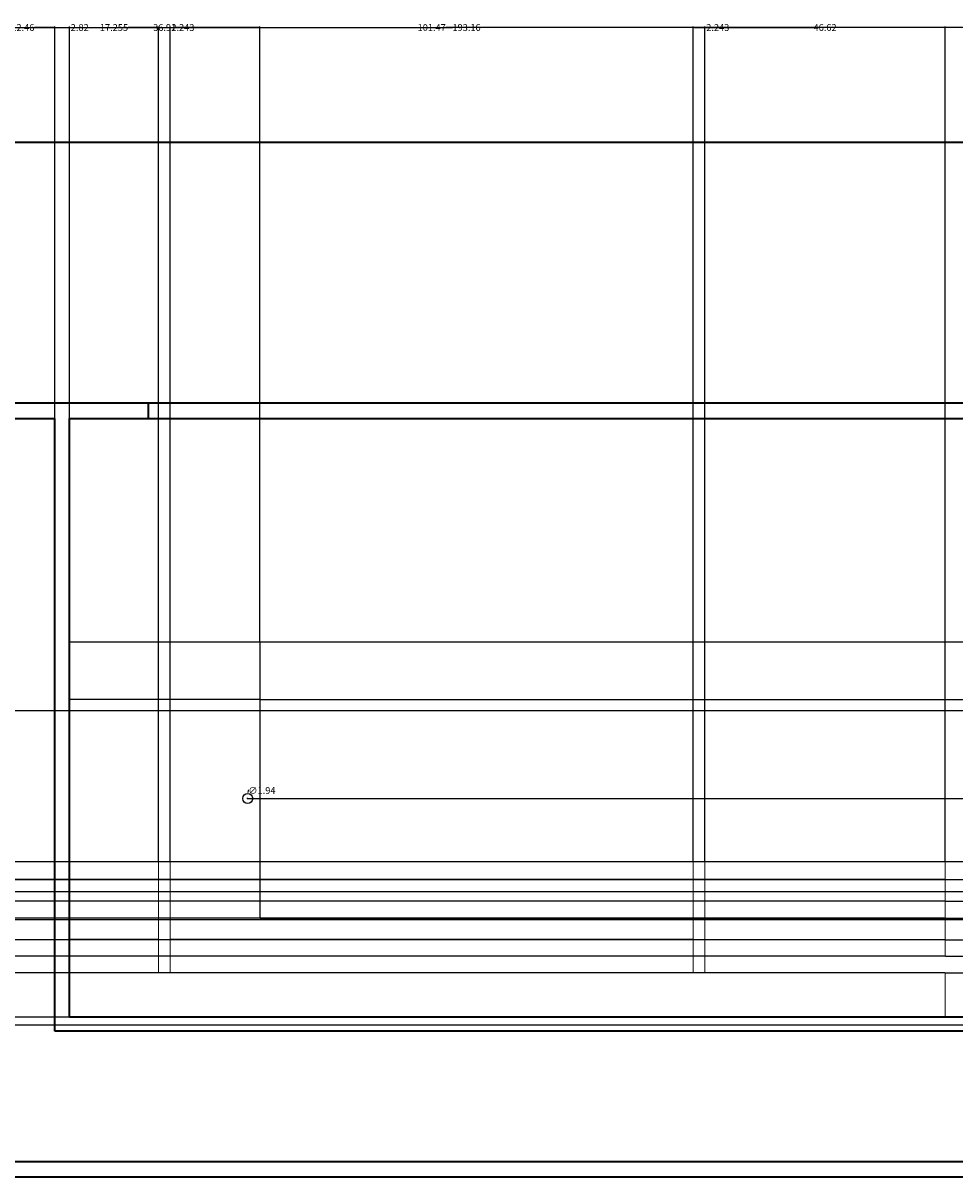
# Model space of a CAD drawing. Units: inches. Extents: x 30 to 515, y 94 to 489.
# Tile 6 of 7: x 202 to 383, y 266 to 489. Entities that reach past the tile are written whole.
import ezdxf

# ---------------------------------------------------------------- set-up
doc = ezdxf.new("R2010")
doc.units = ezdxf.units.IN
doc.header["$MEASUREMENT"] = 0
for name, color, linetype, lineweight in [('A-ANNO-DIMS', 2, 'Continuous', 18), ('A-DOOR', 4, 'Continuous', 25), ('A-FLOR-HRAL', 3, 'Continuous', 18), ('A-ROOF', 1, 'Continuous', 35), ('A-WALL', 7, 'Continuous', 35)]:
    doc.layers.add(name, color=color, linetype=linetype, lineweight=lineweight)
doc.styles.get("Standard").update_dxf_attribs({"font": 'arial.ttf'})
doc.dimstyles.get("Standard").update_dxf_attribs({"dimtxt": 1.3125, "dimasz": 0.18, "dimexe": 0.18, "dimexo": 0.0625, "dimgap": 0.09, "dimtad": 0, "dimtih": 1, "dimtoh": 1, "dimdec": 4, "dimzin": 0, "dimdsep": 46, "dimlunit": 4, "dimtxsty": 'Standard', "dimcen": 0.09, "dimadec": 0, "dimazin": 0, "dimtfac": 1, "dimtdec": 4, "dimtofl": 0, "dimtmove": 0, "dimatfit": 3, "dimfxl": 1, "dimtolj": 1, "dimtzin": 0, "dimarcsym": 0})

# ---------------------------------------------------------------- blocks, each defined once
blk = doc.blocks.new('*D5')
at = {"layer": 'A-ANNO-DIMS', "color": 0, "lineweight": -2, "transparency": 16777216}
for p, q in [((191.21, 466.11), (191.21, 488.48)), ((191.39, 488.3), (285.04, 488.3)), ((384.19, 488.3), (290.54, 488.3)), ((384.37, 466.11), (384.37, 488.48))]:
    blk.add_line(p, q, dxfattribs=at)
at = {"layer": 'A-ANNO-DIMS', "color": 0, "transparency": 16777216}
for points in [[(191.39, 488.33), (191.39, 488.27), (191.21, 488.3)], [(384.19, 488.33), (384.19, 488.27), (384.37, 488.3)]]:
    blk.add_solid(points, dxfattribs=at)
at = {"layer": 'Defpoints', "color": 0, "transparency": 16777216}
for p in [(384.37, 488.3), (191.21, 466.05), (384.37, 466.05)]:
    blk.add_point(p, dxfattribs=at)
at = {"layer": 'A-ANNO-DIMS', "color": 0, "transparency": 16777216, "insert": (287.79, 488.3), "char_height": 1.312, "attachment_point": 5}
blk.add_mtext('\\A1;193.16', dxfattribs=at)
blk = doc.blocks.new('*D30')
at = {"layer": 'A-ANNO-DIMS', "color": 0, "lineweight": -2, "transparency": 16777216}
for p, q in [((210.86, 412.53), (512.17, 412.53)), ((511.99, 412.35), (511.99, 391.63)), ((511.99, 369.4), (511.99, 390.11)), ((247.77, 369.22), (512.17, 369.22))]:
    blk.add_line(p, q, dxfattribs=at)
at = {"layer": 'A-ANNO-DIMS', "color": 0, "transparency": 16777216}
for points in [[(511.96, 412.35), (512.02, 412.35), (511.99, 412.53)], [(511.96, 369.4), (512.02, 369.4), (511.99, 369.22)]]:
    blk.add_solid(points, dxfattribs=at)
at = {"layer": 'Defpoints', "color": 0, "transparency": 16777216}
for p in [(210.8, 412.53), (511.99, 412.53), (247.71, 369.22)]:
    blk.add_point(p, dxfattribs=at)
at = {"layer": 'A-ANNO-DIMS', "color": 0, "transparency": 16777216, "insert": (511.99, 390.87), "char_height": 1.312, "attachment_point": 5}
blk.add_mtext('\\A1;43.31', dxfattribs=at)
blk = doc.blocks.new('*D39')
at = {"layer": 'A-ANNO-DIMS', "color": 0, "lineweight": -2, "transparency": 16777216}
for p, q in [((195.53, 389.32), (195.53, 488.48)), ((195.71, 488.3), (199.51, 488.3)), ((207.81, 488.3), (204, 488.3)), ((207.99, 412.59), (207.99, 488.48))]:
    blk.add_line(p, q, dxfattribs=at)
at = {"layer": 'A-ANNO-DIMS', "color": 0, "transparency": 16777216}
for points in [[(195.71, 488.33), (195.71, 488.27), (195.53, 488.3)], [(207.81, 488.33), (207.81, 488.27), (207.99, 488.3)]]:
    blk.add_solid(points, dxfattribs=at)
at = {"layer": 'Defpoints', "color": 0, "transparency": 16777216}
for p in [(207.99, 488.3), (207.99, 412.53), (195.53, 389.26)]:
    blk.add_point(p, dxfattribs=at)
at = {"layer": 'A-ANNO-DIMS', "color": 0, "transparency": 16777216, "insert": (201.76, 488.3), "char_height": 1.312, "attachment_point": 5}
blk.add_mtext('\\A1;12.46', dxfattribs=at)
blk = doc.blocks.new('*D40')
at = {"layer": 'A-ANNO-DIMS', "color": 0, "lineweight": -2, "transparency": 16777216}
for p, q in [((207.99, 412.59), (207.99, 488.48)), ((208.17, 488.3), (210.62, 488.3)), ((210.8, 412.59), (210.8, 488.48)), ((210.8, 488.3), (210.98, 488.3))]:
    blk.add_line(p, q, dxfattribs=at)
at = {"layer": 'A-ANNO-DIMS', "color": 0, "transparency": 16777216}
for points in [[(208.17, 488.33), (208.17, 488.27), (207.99, 488.3)], [(210.62, 488.33), (210.62, 488.27), (210.8, 488.3)]]:
    blk.add_solid(points, dxfattribs=at)
at = {"layer": 'Defpoints', "color": 0, "transparency": 16777216}
for p in [(210.8, 488.3), (207.99, 412.53), (210.8, 412.53)]:
    blk.add_point(p, dxfattribs=at)
at = {"layer": 'A-ANNO-DIMS', "color": 0, "transparency": 16777216, "insert": (212.78, 488.3), "char_height": 1.312, "attachment_point": 5}
blk.add_mtext('\\A1;2.82', dxfattribs=at)
blk = doc.blocks.new('*D59')
at = {"layer": 'A-ANNO-DIMS', "color": 0, "lineweight": -2, "transparency": 16777216}
for p, q in [((193.04, 296.55), (512.17, 296.55)), ((511.99, 296.73), (511.99, 296.91)), ((195.76, 295.02), (512.17, 295.02)), ((511.99, 294.84), (511.99, 294.66))]:
    blk.add_line(p, q, dxfattribs=at)
at = {"layer": 'A-ANNO-DIMS', "color": 0, "transparency": 16777216}
for points in [[(511.96, 296.73), (512.02, 296.73), (511.99, 296.55)], [(511.96, 294.84), (512.02, 294.84), (511.99, 295.02)]]:
    blk.add_solid(points, dxfattribs=at)
at = {"layer": 'Defpoints', "color": 0, "transparency": 16777216}
for p in [(192.98, 296.55), (511.99, 296.55), (195.7, 295.02)]:
    blk.add_point(p, dxfattribs=at)
at = {"layer": 'A-ANNO-DIMS', "color": 0, "transparency": 16777216, "insert": (511.99, 295.78), "char_height": 1.312, "attachment_point": 5}
blk.add_mtext('\\A1;1.53', dxfattribs=at)
blk = doc.blocks.new('*D60')
at = {"layer": 'A-ANNO-DIMS', "color": 0, "lineweight": -2, "transparency": 16777216}
for p, q in [((191.31, 320.83), (512.17, 320.83)), ((511.99, 320.65), (511.99, 309.45)), ((511.99, 296.73), (511.99, 307.93)), ((193.04, 296.55), (512.17, 296.55))]:
    blk.add_line(p, q, dxfattribs=at)
at = {"layer": 'A-ANNO-DIMS', "color": 0, "transparency": 16777216}
for points in [[(511.96, 320.65), (512.02, 320.65), (511.99, 320.83)], [(511.96, 296.73), (512.02, 296.73), (511.99, 296.55)]]:
    blk.add_solid(points, dxfattribs=at)
at = {"layer": 'Defpoints', "color": 0, "transparency": 16777216}
for p in [(191.25, 320.83), (511.99, 320.83), (192.98, 296.55)]:
    blk.add_point(p, dxfattribs=at)
at = {"layer": 'A-ANNO-DIMS', "color": 0, "transparency": 16777216, "insert": (511.99, 308.69), "char_height": 1.312, "attachment_point": 5}
blk.add_mtext('\\A1;24.275', dxfattribs=at)
blk = doc.blocks.new('*D61')
at = {"layer": 'A-ANNO-DIMS', "color": 0, "lineweight": -2, "transparency": 16777216}
for p, q in [((193.04, 355.95), (512.17, 355.95)), ((511.99, 355.77), (511.99, 339.15)), ((511.99, 321.01), (511.99, 337.63)), ((191.31, 320.83), (512.17, 320.83))]:
    blk.add_line(p, q, dxfattribs=at)
at = {"layer": 'A-ANNO-DIMS', "color": 0, "transparency": 16777216}
for points in [[(511.96, 355.77), (512.02, 355.77), (511.99, 355.95)], [(511.96, 321.01), (512.02, 321.01), (511.99, 320.83)]]:
    blk.add_solid(points, dxfattribs=at)
at = {"layer": 'Defpoints', "color": 0, "transparency": 16777216}
for p in [(192.98, 355.95), (511.99, 355.95), (191.25, 320.83)]:
    blk.add_point(p, dxfattribs=at)
at = {"layer": 'A-ANNO-DIMS', "color": 0, "transparency": 16777216, "insert": (511.99, 338.39), "char_height": 1.312, "attachment_point": 5}
blk.add_mtext('\\A1;35.13', dxfattribs=at)
blk = doc.blocks.new('*D62')
at = {"layer": 'A-ANNO-DIMS', "color": 0, "lineweight": -2, "transparency": 16777216}
for p, q in [((195.76, 315.42), (512.17, 315.42)), ((511.99, 315.24), (511.99, 305.98)), ((511.99, 295.2), (511.99, 304.46)), ((195.76, 295.02), (512.17, 295.02))]:
    blk.add_line(p, q, dxfattribs=at)
at = {"layer": 'A-ANNO-DIMS', "color": 0, "transparency": 16777216}
for points in [[(511.96, 315.24), (512.02, 315.24), (511.99, 315.42)], [(511.96, 295.2), (512.02, 295.2), (511.99, 295.02)]]:
    blk.add_solid(points, dxfattribs=at)
at = {"layer": 'Defpoints', "color": 0, "transparency": 16777216}
for p in [(195.7, 315.42), (511.99, 315.42), (195.7, 295.02)]:
    blk.add_point(p, dxfattribs=at)
at = {"layer": 'A-ANNO-DIMS', "color": 0, "transparency": 16777216, "insert": (511.99, 305.22), "char_height": 1.312, "attachment_point": 5}
blk.add_mtext('\\A1;20.4', dxfattribs=at)
blk = doc.blocks.new('*D63')
at = {"layer": 'A-ANNO-DIMS', "color": 0, "lineweight": -2, "transparency": 16777216}
for p, q in [((195.76, 323.16), (512.17, 323.16)), ((511.99, 322.98), (511.99, 320.04)), ((511.99, 315.6), (511.99, 318.54)), ((195.76, 315.42), (512.17, 315.42))]:
    blk.add_line(p, q, dxfattribs=at)
at = {"layer": 'A-ANNO-DIMS', "color": 0, "transparency": 16777216}
for points in [[(511.96, 322.98), (512.02, 322.98), (511.99, 323.16)], [(511.96, 315.6), (512.02, 315.6), (511.99, 315.42)]]:
    blk.add_solid(points, dxfattribs=at)
at = {"layer": 'Defpoints', "color": 0, "transparency": 16777216}
for p in [(195.7, 323.16), (511.99, 323.16), (195.7, 315.42)]:
    blk.add_point(p, dxfattribs=at)
at = {"layer": 'A-ANNO-DIMS', "color": 0, "transparency": 16777216, "insert": (511.99, 319.29), "char_height": 1.312, "attachment_point": 5}
blk.add_mtext('\\A1;7.74', dxfattribs=at)
blk = doc.blocks.new('*D64')
at = {"layer": 'A-ANNO-DIMS', "color": 0, "lineweight": -2, "transparency": 16777216}
for p, q in [((195.76, 326.67), (512.17, 326.67)), ((511.99, 326.49), (511.99, 325.68)), ((195.76, 323.16), (512.17, 323.16)), ((511.99, 323.34), (511.99, 324.16))]:
    blk.add_line(p, q, dxfattribs=at)
at = {"layer": 'A-ANNO-DIMS', "color": 0, "transparency": 16777216}
for points in [[(511.96, 326.49), (512.02, 326.49), (511.99, 326.67)], [(511.96, 323.34), (512.02, 323.34), (511.99, 323.16)]]:
    blk.add_solid(points, dxfattribs=at)
at = {"layer": 'Defpoints', "color": 0, "transparency": 16777216}
for p in [(195.7, 326.67), (511.99, 326.67), (195.7, 323.16)]:
    blk.add_point(p, dxfattribs=at)
at = {"layer": 'A-ANNO-DIMS', "color": 0, "transparency": 16777216, "insert": (511.99, 324.92), "char_height": 1.312, "attachment_point": 5}
blk.add_mtext('\\A1;3.511', dxfattribs=at)
blk = doc.blocks.new('*D65')
at = {"layer": 'A-ANNO-DIMS', "color": 0, "lineweight": -2, "transparency": 16777216}
for p, q in [((210.8, 369.28), (210.8, 488.48)), ((210.98, 488.3), (227.08, 488.3)), ((247.53, 488.3), (231.43, 488.3)), ((247.71, 369.28), (247.71, 488.48))]:
    blk.add_line(p, q, dxfattribs=at)
at = {"layer": 'A-ANNO-DIMS', "color": 0, "transparency": 16777216}
for points in [[(210.98, 488.33), (210.98, 488.27), (210.8, 488.3)], [(247.53, 488.33), (247.53, 488.27), (247.71, 488.3)]]:
    blk.add_solid(points, dxfattribs=at)
at = {"layer": 'Defpoints', "color": 0, "transparency": 16777216}
for p in [(247.71, 488.3), (210.8, 369.22), (247.71, 369.22)]:
    blk.add_point(p, dxfattribs=at)
at = {"layer": 'A-ANNO-DIMS', "color": 0, "transparency": 16777216, "insert": (229.26, 488.3), "char_height": 1.312, "attachment_point": 5}
blk.add_mtext('\\A1;36.91', dxfattribs=at)
blk = doc.blocks.new('*D66')
at = {"layer": 'A-ANNO-DIMS', "color": 0, "lineweight": -2, "transparency": 16777216}
for p, q in [((210.8, 326.73), (210.8, 488.48)), ((210.98, 488.3), (216.67, 488.3)), ((227.88, 488.3), (222.19, 488.3)), ((228.06, 326.73), (228.06, 488.48))]:
    blk.add_line(p, q, dxfattribs=at)
at = {"layer": 'A-ANNO-DIMS', "color": 0, "transparency": 16777216}
for points in [[(210.98, 488.33), (210.98, 488.27), (210.8, 488.3)], [(227.88, 488.33), (227.88, 488.27), (228.06, 488.3)]]:
    blk.add_solid(points, dxfattribs=at)
at = {"layer": 'Defpoints', "color": 0, "transparency": 16777216}
for p in [(228.06, 488.3), (210.8, 326.67), (228.06, 326.67)]:
    blk.add_point(p, dxfattribs=at)
at = {"layer": 'A-ANNO-DIMS', "color": 0, "transparency": 16777216, "insert": (219.43, 488.3), "char_height": 1.312, "attachment_point": 5}
blk.add_mtext('\\A1;17.255', dxfattribs=at)
blk = doc.blocks.new('*D67')
at = {"layer": 'A-ANNO-DIMS', "color": 0, "lineweight": -2, "transparency": 16777216}
for p, q in [((228.06, 326.73), (228.06, 488.48)), ((228.24, 488.3), (230.12, 488.3)), ((230.3, 326.73), (230.3, 488.48)), ((230.3, 488.3), (230.48, 488.3))]:
    blk.add_line(p, q, dxfattribs=at)
at = {"layer": 'A-ANNO-DIMS', "color": 0, "transparency": 16777216}
for points in [[(228.24, 488.33), (228.24, 488.27), (228.06, 488.3)], [(230.12, 488.33), (230.12, 488.27), (230.3, 488.3)]]:
    blk.add_solid(points, dxfattribs=at)
at = {"layer": 'Defpoints', "color": 0, "transparency": 16777216}
for p in [(230.3, 488.3), (228.06, 326.67), (230.3, 326.67)]:
    blk.add_point(p, dxfattribs=at)
at = {"layer": 'A-ANNO-DIMS', "color": 0, "transparency": 16777216, "insert": (232.79, 488.3), "char_height": 1.312, "attachment_point": 5}
blk.add_mtext('\\A1;2.243', dxfattribs=at)
blk = doc.blocks.new('*D68')
at = {"layer": 'A-ANNO-DIMS', "color": 0, "lineweight": -2, "transparency": 16777216}
for p, q in [((230.3, 326.73), (230.3, 488.48)), ((230.48, 488.3), (278.28, 488.3)), ((331.59, 488.3), (283.79, 488.3)), ((331.77, 326.73), (331.77, 488.48))]:
    blk.add_line(p, q, dxfattribs=at)
at = {"layer": 'A-ANNO-DIMS', "color": 0, "transparency": 16777216}
for points in [[(230.48, 488.33), (230.48, 488.27), (230.3, 488.3)], [(331.59, 488.33), (331.59, 488.27), (331.77, 488.3)]]:
    blk.add_solid(points, dxfattribs=at)
at = {"layer": 'Defpoints', "color": 0, "transparency": 16777216}
for p in [(331.77, 488.3), (230.3, 326.67), (331.77, 326.67)]:
    blk.add_point(p, dxfattribs=at)
at = {"layer": 'A-ANNO-DIMS', "color": 0, "transparency": 16777216, "insert": (281.04, 488.3), "char_height": 1.312, "attachment_point": 5}
blk.add_mtext('\\A1;101.47', dxfattribs=at)
blk = doc.blocks.new('*D69')
at = {"layer": 'A-ANNO-DIMS', "color": 0, "lineweight": -2, "transparency": 16777216}
for p, q in [((331.77, 326.73), (331.77, 488.48)), ((331.95, 488.3), (333.83, 488.3)), ((334.01, 326.73), (334.01, 488.48)), ((334.01, 488.3), (334.19, 488.3))]:
    blk.add_line(p, q, dxfattribs=at)
at = {"layer": 'A-ANNO-DIMS', "color": 0, "transparency": 16777216}
for points in [[(331.95, 488.33), (331.95, 488.27), (331.77, 488.3)], [(333.83, 488.33), (333.83, 488.27), (334.01, 488.3)]]:
    blk.add_solid(points, dxfattribs=at)
at = {"layer": 'Defpoints', "color": 0, "transparency": 16777216}
for p in [(334.01, 488.3), (331.77, 326.67), (334.01, 326.67)]:
    blk.add_point(p, dxfattribs=at)
at = {"layer": 'A-ANNO-DIMS', "color": 0, "transparency": 16777216, "insert": (336.51, 488.3), "char_height": 1.312, "attachment_point": 5}
blk.add_mtext('\\A1;2.243', dxfattribs=at)
blk = doc.blocks.new('*D70')
at = {"layer": 'A-ANNO-DIMS', "color": 0, "lineweight": -2, "transparency": 16777216}
for p, q in [((334.01, 326.73), (334.01, 488.48)), ((334.19, 488.3), (355, 488.3)), ((380.45, 488.3), (359.65, 488.3)), ((380.63, 326.73), (380.63, 488.48))]:
    blk.add_line(p, q, dxfattribs=at)
at = {"layer": 'A-ANNO-DIMS', "color": 0, "transparency": 16777216}
for points in [[(334.19, 488.33), (334.19, 488.27), (334.01, 488.3)], [(380.45, 488.33), (380.45, 488.27), (380.63, 488.3)]]:
    blk.add_solid(points, dxfattribs=at)
at = {"layer": 'Defpoints', "color": 0, "transparency": 16777216}
for p in [(380.63, 488.3), (334.01, 326.67), (380.63, 326.67)]:
    blk.add_point(p, dxfattribs=at)
at = {"layer": 'A-ANNO-DIMS', "color": 0, "transparency": 16777216, "insert": (357.32, 488.3), "char_height": 1.312, "attachment_point": 5}
blk.add_mtext('\\A1;46.62', dxfattribs=at)
blk = doc.blocks.new('*D71')
at = {"layer": 'A-ANNO-DIMS', "color": 0, "lineweight": -2, "transparency": 16777216}
for p, q in [((380.69, 305.1), (512.17, 305.1)), ((511.99, 304.92), (511.99, 301.56)), ((511.99, 296.69), (511.99, 300.04)), ((380.69, 296.51), (512.17, 296.51))]:
    blk.add_line(p, q, dxfattribs=at)
at = {"layer": 'A-ANNO-DIMS', "color": 0, "transparency": 16777216}
for points in [[(511.96, 304.92), (512.02, 304.92), (511.99, 305.1)], [(511.96, 296.69), (512.02, 296.69), (511.99, 296.51)]]:
    blk.add_solid(points, dxfattribs=at)
at = {"layer": 'Defpoints', "color": 0, "transparency": 16777216}
for p in [(380.63, 305.1), (511.99, 305.1), (380.63, 296.51)]:
    blk.add_point(p, dxfattribs=at)
at = {"layer": 'A-ANNO-DIMS', "color": 0, "transparency": 16777216, "insert": (511.99, 300.8), "char_height": 1.312, "attachment_point": 5}
blk.add_mtext('\\A1;8.585', dxfattribs=at)
blk = doc.blocks.new('*D72')
at = {"layer": 'A-ANNO-DIMS', "color": 0, "lineweight": -2, "transparency": 16777216}
for p, q in [((380.69, 311.45), (512.17, 311.45)), ((511.99, 311.27), (511.99, 310.65)), ((511.99, 308.51), (511.99, 309.13)), ((380.69, 308.33), (512.17, 308.33))]:
    blk.add_line(p, q, dxfattribs=at)
at = {"layer": 'A-ANNO-DIMS', "color": 0, "transparency": 16777216}
for points in [[(511.96, 311.27), (512.02, 311.27), (511.99, 311.45)], [(511.96, 308.51), (512.02, 308.51), (511.99, 308.33)]]:
    blk.add_solid(points, dxfattribs=at)
at = {"layer": 'Defpoints', "color": 0, "transparency": 16777216}
for p in [(380.63, 311.45), (511.99, 311.45), (380.63, 308.33)]:
    blk.add_point(p, dxfattribs=at)
at = {"layer": 'A-ANNO-DIMS', "color": 0, "transparency": 16777216, "insert": (511.99, 309.89), "char_height": 1.312, "attachment_point": 5}
blk.add_mtext('\\A1;3.117', dxfattribs=at)
blk = doc.blocks.new('*D73')
at = {"layer": 'A-ANNO-DIMS', "color": 0, "lineweight": -2, "transparency": 16777216}
for p, q in [((380.69, 319), (512.17, 319)), ((511.99, 318.82), (511.99, 318.11)), ((380.69, 315.69), (512.17, 315.69)), ((511.99, 315.87), (511.99, 316.59))]:
    blk.add_line(p, q, dxfattribs=at)
at = {"layer": 'A-ANNO-DIMS', "color": 0, "transparency": 16777216}
for points in [[(511.96, 318.82), (512.02, 318.82), (511.99, 319)], [(511.96, 315.87), (512.02, 315.87), (511.99, 315.69)]]:
    blk.add_solid(points, dxfattribs=at)
at = {"layer": 'Defpoints', "color": 0, "transparency": 16777216}
for p in [(380.63, 319), (511.99, 319), (380.63, 315.69)]:
    blk.add_point(p, dxfattribs=at)
at = {"layer": 'A-ANNO-DIMS', "color": 0, "transparency": 16777216, "insert": (511.99, 317.35), "char_height": 1.312, "attachment_point": 5}
blk.add_mtext('\\A1;3.31', dxfattribs=at)
blk = doc.blocks.new('*D74')
at = {"layer": 'A-ANNO-DIMS', "color": 0, "lineweight": -2, "transparency": 16777216}
for p, q in [((380.69, 326.67), (512.17, 326.67)), ((511.99, 326.49), (511.99, 325.68)), ((380.69, 323.16), (512.17, 323.16)), ((511.99, 323.34), (511.99, 324.16))]:
    blk.add_line(p, q, dxfattribs=at)
at = {"layer": 'A-ANNO-DIMS', "color": 0, "transparency": 16777216}
for points in [[(511.96, 326.49), (512.02, 326.49), (511.99, 326.67)], [(511.96, 323.34), (512.02, 323.34), (511.99, 323.16)]]:
    blk.add_solid(points, dxfattribs=at)
at = {"layer": 'Defpoints', "color": 0, "transparency": 16777216}
for p in [(380.63, 326.67), (511.99, 326.67), (380.63, 323.16)]:
    blk.add_point(p, dxfattribs=at)
at = {"layer": 'A-ANNO-DIMS', "color": 0, "transparency": 16777216, "insert": (511.99, 324.92), "char_height": 1.312, "attachment_point": 5}
blk.add_mtext('\\A1;3.511', dxfattribs=at)
blk = doc.blocks.new('*D75')
at = {"layer": 'A-ANNO-DIMS', "color": 0, "lineweight": -2, "transparency": 16777216}
for p, q in [((380.57, 308.33), (32.48, 308.33)), ((32.66, 308.15), (32.66, 307.47)), ((380.57, 305.1), (32.48, 305.1)), ((32.66, 305.28), (32.66, 305.95))]:
    blk.add_line(p, q, dxfattribs=at)
at = {"layer": 'A-ANNO-DIMS', "color": 0, "transparency": 16777216}
for points in [[(32.63, 308.15), (32.69, 308.15), (32.66, 308.33)], [(32.63, 305.28), (32.69, 305.28), (32.66, 305.1)]]:
    blk.add_solid(points, dxfattribs=at)
at = {"layer": 'Defpoints', "color": 0, "transparency": 16777216}
for p in [(32.66, 308.33), (380.63, 308.33), (380.63, 305.1)]:
    blk.add_point(p, dxfattribs=at)
at = {"layer": 'A-ANNO-DIMS', "color": 0, "transparency": 16777216, "insert": (32.66, 306.71), "char_height": 1.312, "attachment_point": 5}
blk.add_mtext('\\A1;3.238', dxfattribs=at)
blk = doc.blocks.new('*D76')
at = {"layer": 'A-ANNO-DIMS', "color": 0, "lineweight": -2, "transparency": 16777216}
for p, q in [((380.57, 315.69), (32.48, 315.69)), ((32.66, 315.51), (32.66, 314.33)), ((380.57, 311.45), (32.48, 311.45)), ((32.66, 311.63), (32.66, 312.81))]:
    blk.add_line(p, q, dxfattribs=at)
at = {"layer": 'A-ANNO-DIMS', "color": 0, "transparency": 16777216}
for points in [[(32.63, 315.51), (32.69, 315.51), (32.66, 315.69)], [(32.63, 311.63), (32.69, 311.63), (32.66, 311.45)]]:
    blk.add_solid(points, dxfattribs=at)
at = {"layer": 'Defpoints', "color": 0, "transparency": 16777216}
for p in [(32.66, 315.69), (380.63, 315.69), (380.63, 311.45)]:
    blk.add_point(p, dxfattribs=at)
at = {"layer": 'A-ANNO-DIMS', "color": 0, "transparency": 16777216, "insert": (32.66, 313.57), "char_height": 1.312, "attachment_point": 5}
blk.add_mtext('\\A1;4.243', dxfattribs=at)
blk = doc.blocks.new('*D77')
at = {"layer": 'A-ANNO-DIMS', "color": 0, "lineweight": -2, "transparency": 16777216}
for p, q in [((380.57, 323.16), (32.48, 323.16)), ((32.66, 322.98), (32.66, 321.84)), ((32.66, 319.18), (32.66, 320.32)), ((380.57, 319), (32.48, 319))]:
    blk.add_line(p, q, dxfattribs=at)
at = {"layer": 'A-ANNO-DIMS', "color": 0, "transparency": 16777216}
for points in [[(32.63, 322.98), (32.69, 322.98), (32.66, 323.16)], [(32.63, 319.18), (32.69, 319.18), (32.66, 319)]]:
    blk.add_solid(points, dxfattribs=at)
at = {"layer": 'Defpoints', "color": 0, "transparency": 16777216}
for p in [(32.66, 323.16), (380.63, 323.16), (380.63, 319)]:
    blk.add_point(p, dxfattribs=at)
at = {"layer": 'A-ANNO-DIMS', "color": 0, "transparency": 16777216, "insert": (32.66, 321.08), "char_height": 1.312, "attachment_point": 5}
blk.add_mtext('\\A1;4.16', dxfattribs=at)
blk = doc.blocks.new('*D78')
at = {"layer": 'A-ANNO-DIMS', "color": 0, "lineweight": -2, "transparency": 16777216}
for p, q in [((245.42, 338.88), (512.17, 338.88)), ((511.99, 338.7), (511.99, 328.05)), ((511.99, 315.87), (511.99, 326.52)), ((247.77, 315.69), (512.17, 315.69))]:
    blk.add_line(p, q, dxfattribs=at)
at = {"layer": 'A-ANNO-DIMS', "color": 0, "transparency": 16777216}
for points in [[(511.96, 338.7), (512.02, 338.7), (511.99, 338.88)], [(511.96, 315.87), (512.02, 315.87), (511.99, 315.69)]]:
    blk.add_solid(points, dxfattribs=at)
at = {"layer": 'Defpoints', "color": 0, "transparency": 16777216}
for p in [(245.35, 338.88), (511.99, 338.88), (247.71, 315.69)]:
    blk.add_point(p, dxfattribs=at)
at = {"layer": 'A-ANNO-DIMS', "color": 0, "transparency": 16777216, "insert": (511.99, 327.29), "char_height": 1.312, "attachment_point": 5}
blk.add_mtext('\\A1;23.183', dxfattribs=at)
blk = doc.blocks.new('*D79')
at = {"layer": 'A-ANNO-DIMS', "color": 0, "lineweight": -2, "transparency": 16777216}
for p, q in [((247.77, 358.06), (512.17, 358.06)), ((511.99, 357.88), (511.99, 349.23)), ((511.99, 339.06), (511.99, 347.71)), ((245.42, 338.88), (512.17, 338.88))]:
    blk.add_line(p, q, dxfattribs=at)
at = {"layer": 'A-ANNO-DIMS', "color": 0, "transparency": 16777216}
for points in [[(511.96, 357.88), (512.02, 357.88), (511.99, 358.06)], [(511.96, 339.06), (512.02, 339.06), (511.99, 338.88)]]:
    blk.add_solid(points, dxfattribs=at)
at = {"layer": 'Defpoints', "color": 0, "transparency": 16777216}
for p in [(247.71, 358.06), (511.99, 358.06), (245.35, 338.88)]:
    blk.add_point(p, dxfattribs=at)
at = {"layer": 'A-ANNO-DIMS', "color": 0, "transparency": 16777216, "insert": (511.99, 348.47), "char_height": 1.312, "attachment_point": 5}
blk.add_mtext('\\A1;19.184', dxfattribs=at)
blk = doc.blocks.new('*D80')
at = {"layer": 'A-ANNO-DIMS', "color": 0, "lineweight": -2, "transparency": 16777216}
for p, q in [((247.77, 369.22), (512.17, 369.22)), ((511.99, 369.04), (511.99, 364.4)), ((511.99, 358.24), (511.99, 362.88)), ((247.77, 358.06), (512.17, 358.06))]:
    blk.add_line(p, q, dxfattribs=at)
at = {"layer": 'A-ANNO-DIMS', "color": 0, "transparency": 16777216}
for points in [[(511.96, 369.04), (512.02, 369.04), (511.99, 369.22)], [(511.96, 358.24), (512.02, 358.24), (511.99, 358.06)]]:
    blk.add_solid(points, dxfattribs=at)
at = {"layer": 'Defpoints', "color": 0, "transparency": 16777216}
for p in [(247.71, 369.22), (511.99, 369.22), (247.71, 358.06)]:
    blk.add_point(p, dxfattribs=at)
at = {"layer": 'A-ANNO-DIMS', "color": 0, "transparency": 16777216, "insert": (511.99, 363.64), "char_height": 1.312, "attachment_point": 5}
blk.add_mtext('\\A1;11.16', dxfattribs=at)
blk = doc.blocks.new('*D82')
at = {"layer": 'A-ANNO-DIMS', "color": 0, "lineweight": -2, "transparency": 16777216}
for p, q in [((245.42, 340.42), (245.41, 340.02)), ((245.6, 340.42), (245.42, 340.42)), ((245.26, 338.88), (245.44, 338.88)), ((245.35, 338.79), (245.35, 338.97))]:
    blk.add_line(p, q, dxfattribs=at)
at = {"layer": 'A-ANNO-DIMS', "color": 0, "transparency": 16777216}
blk.add_solid([(245.38, 340.02), (245.44, 340.02), (245.4, 339.84)], dxfattribs=at)
at = {"layer": 'Defpoints', "color": 0, "transparency": 16777216}
for p in [(245.31, 337.91), (245.4, 339.84)]:
    blk.add_point(p, dxfattribs=at)
at = {"layer": 'A-ANNO-DIMS', "color": 0, "transparency": 16777216, "insert": (248.11, 340.42), "char_height": 1.312, "attachment_point": 5}
blk.add_mtext('\\A1;∅1.94', dxfattribs=at)

msp = doc.modelspace()

# ---------------------------------------------------------------- linework, layer by layer
at = {"layer": 'A-DOOR'}
for p, q in [((247.7111, 358.0606), (247.7111, 315.6935)), ((247.7111, 315.6935), (210.8018, 315.6935))]:
    msp.add_line(p, q, dxfattribs=at)
msp.add_lwpolyline([(210.8018, 369.2198), (247.7111, 369.2198), (247.7111, 358.0606), (210.8018, 358.0606)], close=True, dxfattribs=at)
msp.add_circle((245.3541, 338.8769), 0.9677, dxfattribs=at)
at = {"layer": 'A-FLOR-HRAL'}
for p, q in [((210.8018, 326.6711), (380.6303, 326.6711)), ((228.0564, 323.1601), (228.0564, 326.6711)), ((230.2993, 323.1601), (230.2993, 326.6711)), ((331.772, 323.1601), (331.772, 326.6711)), ((334.0149, 323.1601), (334.0149, 326.6711)), ((380.6303, 323.1601), (380.6303, 326.6711)), ((210.8018, 323.1601), (380.6303, 323.1601)), ((228.0564, 321.7478), (228.0564, 323.1601)), ((230.2993, 321.7478), (230.2993, 323.1601)), ((331.772, 305.0952), (331.772, 323.1601)), ((334.0149, 323.1601), (334.0149, 305.0952)), ((380.6303, 315.6935), (380.6303, 323.1601)), ((228.0564, 305.0952), (228.0564, 321.7478)), ((230.2993, 321.7478), (230.2993, 305.0952)), ((210.8018, 319.0036), (228.0564, 319.0036)), ((230.2993, 319.0036), (331.772, 319.0036)), ((334.0149, 319.0036), (380.6303, 319.0036)), ((247.7111, 315.6935), (380.6303, 315.6935)), ((380.6303, 308.3335), (380.6303, 315.6935)), ((210.8018, 311.6236), (228.0564, 311.6236)), ((230.2993, 311.6236), (331.772, 311.6236)), ((334.0149, 311.4502), (380.6303, 311.4502)), ((210.8018, 308.3335), (228.0564, 308.3335)), ((230.2993, 308.3335), (380.6303, 308.3335)), ((228.0564, 305.0952), (210.8018, 305.0952)), ((228.0564, 305.0952), (230.2993, 305.0952)), ((230.2993, 305.0952), (331.772, 305.0952)), ((331.772, 305.0952), (380.6303, 305.0952)), ((380.6303, 305.0952), (380.6303, 296.5098))]:
    msp.add_line(p, q, dxfattribs=at)
at = {"layer": 'A-ROOF'}
for p, q in [((191.2145, 466.0503), (286.8264, 466.0503)), ((286.8264, 466.0503), (337.6614, 466.0503)), ((337.6614, 466.0503), (384.3704, 466.0503))]:
    msp.add_line(p, q, dxfattribs=at)
at = {"layer": 'A-WALL'}
for p, q in [((67.017, 415.5281), (448.0511, 415.5281)), ((226.0705, 415.5281), (226.0705, 412.5281)), ((67.017, 412.5281), (207.9863, 412.5281)), ((207.9863, 293.7914), (207.9863, 412.5281)), ((210.8018, 296.5098), (210.8018, 412.5281)), ((210.8018, 412.5281), (448.0511, 412.5281)), ((489.7426, 296.5098), (210.8018, 296.5098)), ((485.0273, 293.7914), (207.9863, 293.7914)), ((67.017, 268.5281), (448.0511, 268.5281)), ((67.017, 265.5281), (448.0511, 265.5281))]:
    msp.add_line(p, q, dxfattribs=at)

# ---------------------------------------------------------------- dimensions: what is measured, and where the dimension line sits
at = {"layer": 'A-ANNO-DIMS'}
for base, p1, p2, override, picture, middle in [((384.3704, 488.3003), (191.2145, 466.0503), (384.3704, 466.0503), {"dimdec": 2, "dimlfac": 1, "dimrnd": 0, "dimzin": 0, "dimdsep": 46, "dimlunit": 2}, '*D5', (287.7924, 488.3003)), ((207.9863, 488.3003), (195.5251, 389.2603), (207.9863, 412.5281), {"dimdec": 2, "dimlfac": 1, "dimrnd": 0, "dimzin": 0, "dimdsep": 46, "dimlunit": 2}, '*D39', (201.7557, 488.3003)), ((210.8018, 488.3003), (207.9863, 412.5281), (210.8018, 412.5281), {"dimdec": 2, "dimlfac": 1, "dimrnd": 0, "dimzin": 0, "dimdsep": 46, "dimlunit": 2}, '*D40', (212.7809, 488.3003)), ((247.7111, 488.3003), (210.8018, 369.2198), (247.7111, 369.2198), {"dimdec": 2, "dimlfac": 1, "dimrnd": 0, "dimzin": 0, "dimdsep": 46, "dimlunit": 2}, '*D65', (229.2565, 488.3003)), ((228.0564, 488.3003), (210.8018, 326.6711), (228.0564, 326.6711), {"dimdec": 3, "dimlfac": 1, "dimrnd": 0, "dimzin": 0, "dimdsep": 46, "dimlunit": 2}, '*D66', (219.4291, 488.3003)), ((230.2993, 488.3003), (228.0564, 326.6711), (230.2993, 326.6711), {"dimdec": 3, "dimlfac": 1, "dimrnd": 0, "dimzin": 0, "dimdsep": 46, "dimlunit": 2}, '*D67', (232.795, 488.3003)), ((331.772, 488.3003), (230.2993, 326.6711), (331.772, 326.6711), {"dimdec": 2, "dimlfac": 1, "dimrnd": 0, "dimzin": 0, "dimdsep": 46, "dimlunit": 2}, '*D68', (281.0356, 488.3003)), ((334.0149, 488.3003), (331.772, 326.6711), (334.0149, 326.6711), {"dimdec": 3, "dimlfac": 1, "dimrnd": 0, "dimzin": 0, "dimdsep": 46, "dimlunit": 2}, '*D69', (336.5106, 488.3003)), ((380.6303, 488.3003), (334.0149, 326.6711), (380.6303, 326.6711), {"dimdec": 2, "dimlfac": 1, "dimrnd": 0, "dimzin": 0, "dimdsep": 46, "dimlunit": 2}, '*D70', (357.3226, 488.3003))]:
    dim = msp.add_linear_dim(base=base, p1=p1, p2=p2, dimstyle='Standard', override=override, dxfattribs=at)
    dim.commit()
    dim.dimension.update_dxf_attribs({"geometry": picture, "text_midpoint": middle})
for base, p1, p2, override, picture, middle in [((511.9926, 412.5281), (247.7111, 369.2198), (210.8018, 412.5281), {"dimdec": 2, "dimlfac": 1, "dimrnd": 0, "dimzin": 0, "dimdsep": 46, "dimlunit": 2}, '*D30', (511.9926, 390.8739)), ((511.9926, 369.2198), (247.7111, 358.0606), (247.7111, 369.2198), {"dimdec": 2, "dimlfac": 1, "dimrnd": 0, "dimzin": 0, "dimdsep": 46, "dimlunit": 2}, '*D80', (511.9926, 363.6402)), ((511.9926, 358.0606), (245.3541, 338.8769), (247.7111, 358.0606), {"dimdec": 3, "dimlfac": 1, "dimrnd": 0, "dimzin": 0, "dimdsep": 46, "dimlunit": 2}, '*D79', (511.9926, 348.4687)), ((511.9926, 355.9547), (191.2506, 320.8262), (192.9806, 355.9547), {"dimdec": 2, "dimlfac": 1, "dimrnd": 0, "dimzin": 0, "dimdsep": 46, "dimlunit": 2}, '*D61', (511.9926, 338.3905)), ((511.9926, 338.8769), (247.7111, 315.6935), (245.3541, 338.8769), {"dimdec": 3, "dimlfac": 1, "dimrnd": 0, "dimzin": 0, "dimdsep": 46, "dimlunit": 2}, '*D78', (511.9926, 327.2852)), ((511.9926, 326.6711), (195.6952, 323.1601), (195.6952, 326.6711), {"dimdec": 3, "dimlfac": 1, "dimrnd": 0, "dimzin": 0, "dimdsep": 46, "dimlunit": 2}, '*D64', (511.9926, 324.9156)), ((511.9926, 326.6711), (380.6303, 323.1601), (380.6303, 326.6711), {"dimdec": 3, "dimlfac": 1, "dimrnd": 0, "dimzin": 0, "dimdsep": 46, "dimlunit": 2}, '*D74', (511.9926, 324.9156)), ((32.6647, 323.1601), (380.6303, 319.0036), (380.6303, 323.1601), {"dimdec": 2, "dimlfac": 1, "dimrnd": 0, "dimzin": 0, "dimdsep": 46, "dimlunit": 2}, '*D77', (32.6647, 321.0818)), ((511.9926, 323.1601), (195.6952, 315.4195), (195.6952, 323.1601), {"dimdec": 2, "dimlfac": 1, "dimrnd": 0, "dimzin": 0, "dimdsep": 46, "dimlunit": 2}, '*D63', (511.9926, 319.2898)), ((511.9926, 320.8262), (192.9806, 296.551), (191.2506, 320.8262), {"dimdec": 3, "dimlfac": 1, "dimrnd": 0, "dimzin": 0, "dimdsep": 46, "dimlunit": 2}, '*D60', (511.9926, 308.6886)), ((511.9926, 319.0036), (380.6303, 315.6935), (380.6303, 319.0036), {"dimdec": 2, "dimlfac": 1, "dimrnd": 0, "dimzin": 0, "dimdsep": 46, "dimlunit": 2}, '*D73', (511.9926, 317.3485)), ((32.6647, 315.6935), (380.6303, 311.4502), (380.6303, 315.6935), {"dimdec": 3, "dimlfac": 1, "dimrnd": 0, "dimzin": 0, "dimdsep": 46, "dimlunit": 2}, '*D76', (32.6647, 313.5719)), ((511.9926, 315.4195), (195.6952, 295.0176), (195.6952, 315.4195), {"dimdec": 1, "dimlfac": 1, "dimrnd": 0, "dimzin": 0, "dimdsep": 46, "dimlunit": 2}, '*D62', (511.9926, 305.2186)), ((511.9926, 311.4502), (380.6303, 308.3335), (380.6303, 311.4502), {"dimdec": 3, "dimlfac": 1, "dimrnd": 0, "dimzin": 0, "dimdsep": 46, "dimlunit": 2}, '*D72', (511.9926, 309.8918)), ((32.6647, 308.3335), (380.6303, 305.0952), (380.6303, 308.3335), {"dimdec": 3, "dimlfac": 1, "dimrnd": 0, "dimzin": 0, "dimdsep": 46, "dimlunit": 2}, '*D75', (32.6647, 306.7144)), ((511.9926, 305.0952), (380.6303, 296.5098), (380.6303, 305.0952), {"dimdec": 3, "dimlfac": 1, "dimrnd": 0, "dimzin": 0, "dimdsep": 46, "dimlunit": 2}, '*D71', (511.9926, 300.8025)), ((511.9926, 296.551), (195.6952, 295.0176), (192.9806, 296.551), {"dimdec": 2, "dimlfac": 1, "dimrnd": 0, "dimzin": 0, "dimdsep": 46, "dimlunit": 2}, '*D59', (511.9926, 295.7843))]:
    dim = msp.add_linear_dim(base=base, p1=p1, p2=p2, angle=90, dimstyle='Standard', override=override, dxfattribs=at)
    dim.commit()
    dim.dimension.update_dxf_attribs({"geometry": picture, "text_midpoint": middle})
dim = msp.add_diameter_dim_2p(p1=(245.3107, 337.9102), p2=(245.3975, 339.8437), dimstyle='Standard', override={"dimdec": 2, "dimlfac": 1, "dimrnd": 0, "dimzin": 0, "dimdsep": 46, "dimlunit": 2}, dxfattribs=at)
dim.commit()
dim.dimension.update_dxf_attribs({"geometry": '*D82', "text_midpoint": (248.1095, 340.4237), "dimtype": 163})

doc.saveas('drawing.dxf')
